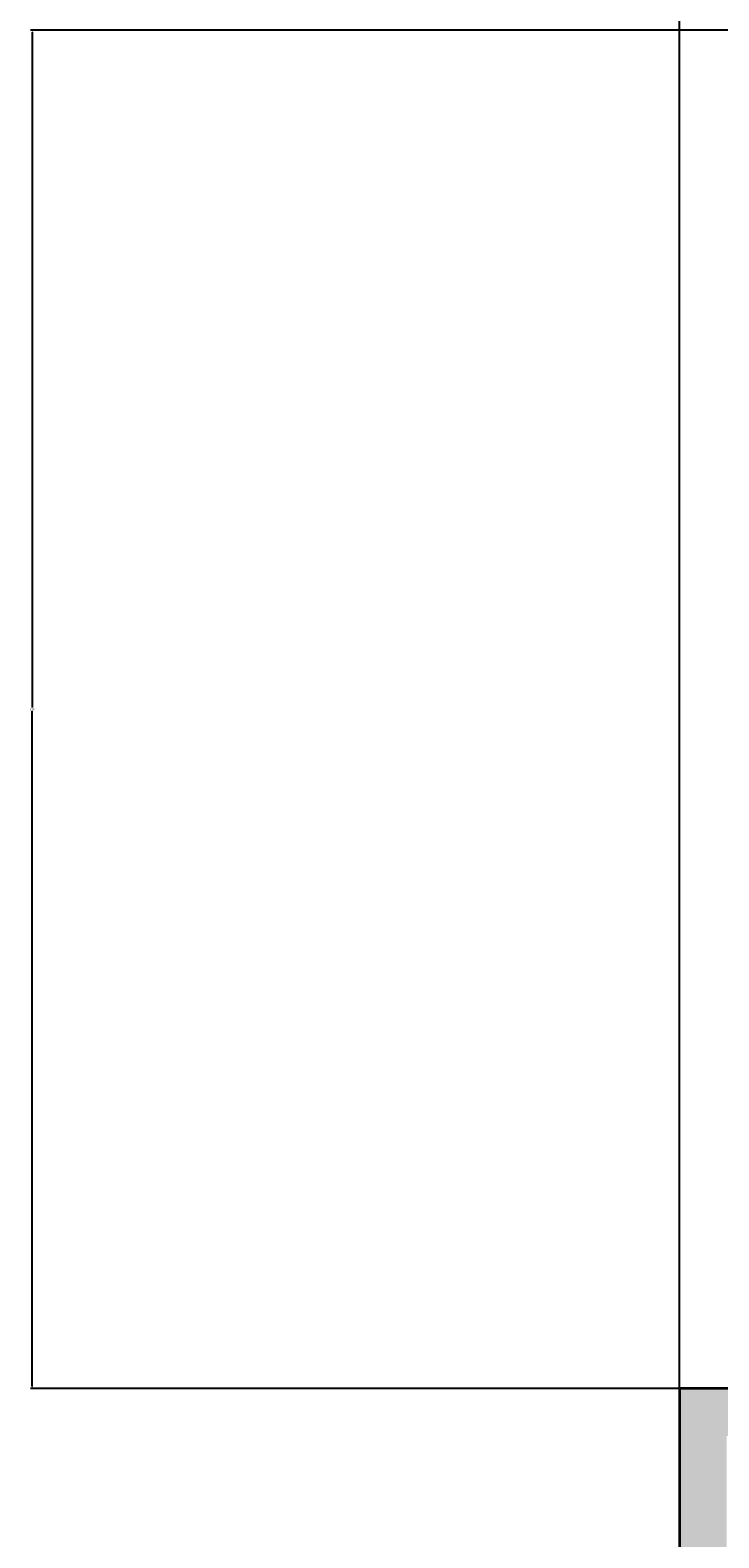
# Model space of a CAD drawing. Units: inches. Extents: x 1998 to 2588, y 1139 to 1977.
# Tile 58 of 134: x 1998 to 2063, y 1746 to 1889. Entities that reach past the tile are written whole.
import ezdxf

# ---------------------------------------------------------------- set-up
doc = ezdxf.new("R2010")
doc.units = ezdxf.units.IN
for name, color, linetype, lineweight in [('A-ANNO-DIMS', 2, 'Continuous', 18), ('A-WALL-PATT', 252, 'Continuous', 13), ('WALL', 200, 'Continuous', 35)]:
    doc.layers.add(name, color=color, linetype=linetype, lineweight=lineweight)
doc.styles.get("Standard").update_dxf_attribs({"font": 'arial.ttf'})
doc.dimstyles.get("Standard").update_dxf_attribs({"dimtxt": 0.18, "dimasz": 0.18, "dimexe": 0.18, "dimexo": 0.0625, "dimgap": 0.09, "dimtad": 0, "dimtih": 1, "dimtoh": 1, "dimdec": 4, "dimzin": 0, "dimdsep": 46, "dimtxsty": 'Standard', "dimcen": 0.09, "dimadec": 0, "dimazin": 0, "dimtfac": 1, "dimtdec": 4, "dimtofl": 0, "dimtmove": 0, "dimatfit": 3, "dimfxl": 1, "dimtolj": 1, "dimtzin": 0, "dimarcsym": 0})

# ---------------------------------------------------------------- blocks, each defined once
blk = doc.blocks.new('*D28')
at = {"layer": 'A-ANNO-DIMS', "color": 0, "lineweight": -2, "transparency": 16777216}
for p, q in [((2059.47, 1759.79), (2059.47, 1977.36)), ((2059.65, 1977.18), (2073.4, 1977.18)), ((2087.79, 1977.18), (2074.05, 1977.18)), ((2087.97, 1759.79), (2087.97, 1977.36))]:
    blk.add_line(p, q, dxfattribs=at)
at = {"layer": 'A-ANNO-DIMS', "color": 0, "transparency": 16777216}
for points in [[(2059.65, 1977.21), (2059.65, 1977.15), (2059.47, 1977.18)], [(2087.79, 1977.21), (2087.79, 1977.15), (2087.97, 1977.18)]]:
    blk.add_solid(points, dxfattribs=at)
at = {"layer": 'Defpoints', "color": 0, "transparency": 16777216}
for p in [(2087.97, 1977.18), (2059.47, 1759.73), (2087.97, 1759.73)]:
    blk.add_point(p, dxfattribs=at)
at = {"layer": 'A-ANNO-DIMS', "color": 0, "transparency": 16777216, "insert": (2073.72, 1977.18), "char_height": 0.18, "attachment_point": 5}
blk.add_mtext('\\A1;28.5', dxfattribs=at)
blk = doc.blocks.new('*D29')
at = {"layer": 'A-ANNO-DIMS', "color": 0, "lineweight": -2, "transparency": 16777216}
for p, q in [((2087.91, 1888.73), (1997.84, 1888.73)), ((1998.02, 1888.55), (1998.02, 1824.41)), ((1998.02, 1759.91), (1998.02, 1824.05)), ((2059.41, 1759.73), (1997.84, 1759.73))]:
    blk.add_line(p, q, dxfattribs=at)
at = {"layer": 'A-ANNO-DIMS', "color": 0, "transparency": 16777216}
for points in [[(1997.99, 1888.55), (1998.05, 1888.55), (1998.02, 1888.73)], [(1997.99, 1759.91), (1998.05, 1759.91), (1998.02, 1759.73)]]:
    blk.add_solid(points, dxfattribs=at)
at = {"layer": 'Defpoints', "color": 0, "transparency": 16777216}
for p in [(1998.02, 1888.73), (2087.97, 1888.73), (2059.47, 1759.73)]:
    blk.add_point(p, dxfattribs=at)
at = {"layer": 'A-ANNO-DIMS', "color": 0, "transparency": 16777216, "insert": (1998.02, 1824.23), "char_height": 0.18, "attachment_point": 5}
blk.add_mtext('\\A1;129', dxfattribs=at)

msp = doc.modelspace()

# ---------------------------------------------------------------- hatches: boundary and pattern name
at = {"layer": 'A-WALL-PATT'}
h = msp.add_hatch(color=256, dxfattribs=at)
h.dxf.hatch_style = 1
h.paths.add_polyline_path([(2222.9729, 1888.7324), (2099.4125, 1888.7324), (2099.4125, 1879.7324), (2222.9729, 1879.7324)])
h.paths.add_polyline_path([(2096.9729, 1868.3278), (2087.9729, 1868.3278), (2087.9729, 1775.637), (2096.9729, 1775.637)])
h.paths.add_polyline_path([(2227.4729, 1868.3278), (2222.9729, 1868.3278), (2222.9729, 1774.3318), (2227.4729, 1774.3318)])
h.paths.add_polyline_path([(2188.3019, 1759.7324), (2138.6074, 1759.7324), (2099.4125, 1759.7324), (2099.4125, 1755.2324), (2176.9729, 1755.2324), (2188.3019, 1755.2324)])
h.paths.add_polyline_path([(2087.9729, 1759.7324), (2059.4729, 1759.7324), (2059.4729, 1702.7324), (2087.9729, 1702.7324), (2087.9729, 1707.2324), (2063.9729, 1707.2324), (2063.9729, 1755.2324), (2087.9729, 1755.2324)])
h.paths.add_polyline_path([(2096.9729, 1755.2324), (2087.9729, 1755.2324), (2087.9729, 1707.2324), (2096.9729, 1707.2324)])
h.paths.add_polyline_path([(2187.0461, 1707.2324), (2105.9729, 1707.2324), (2096.9729, 1707.2324), (2087.9729, 1707.2324), (2087.9729, 1702.7324), (2105.9729, 1702.7324), (2114.9729, 1702.7324), (2187.0461, 1702.7324)])
h.paths.add_polyline_path([(2181.4729, 1719.2028), (2176.9729, 1719.2028), (2176.9729, 1707.2324), (2181.4729, 1707.2324)])
h.paths.add_polyline_path([(2216.0332, 1588.7324), (2114.9729, 1588.7324), (2105.9729, 1588.7324), (2105.9729, 1584.2324), (2216.0332, 1584.2324)])
h.paths.add_polyline_path([(2077.691, 1588.7324), (2061.4729, 1588.7324), (2061.4729, 1584.2324), (2077.691, 1584.2324)])
h.paths.add_polyline_path([(2105.9729, 1588.7324), (2098.0956, 1588.7324), (2098.0956, 1584.2324), (2105.9729, 1584.2324)])
h.paths.add_polyline_path([(2114.9729, 1596.2642), (2110.1012, 1596.2642), (2105.9729, 1596.2642), (2105.9729, 1588.7324), (2114.9729, 1588.7324)])
h.paths.add_polyline_path([(2114.9729, 1584.2324), (2105.9729, 1584.2324), (2105.9729, 1580.249), (2110.1012, 1580.249), (2114.9729, 1580.249)])
h.paths.add_polyline_path([(2114.9729, 1547.7716), (2110.1012, 1547.7716, -0.0318759), (2105.9729, 1548.035), (2105.9729, 1470.2324), (2108.3775, 1470.2324), (2108.3775, 1465.7324), (2186.2943, 1465.7324), (2186.2943, 1470.2324), (2114.9729, 1470.2324)])
h.paths.add_polyline_path([(2227.4729, 1584.2324), (2222.9729, 1584.2324), (2222.9729, 1486.137), (2227.4729, 1486.137)])
h.paths.add_polyline_path([(2295.4138, 1593.2324), (2227.4729, 1593.2324), (2227.4729, 1588.7324), (2295.4138, 1588.7324), (2295.4138, 1591.8729)])
h.paths.add_polyline_path([(2345.9729, 1627.1165), (2341.4729, 1627.1165), (2341.4729, 1593.2324), (2337.2869, 1593.2324), (2337.2869, 1591.8729), (2337.2869, 1588.7324), (2345.9729, 1588.7324)])
h.paths.add_polyline_path([(2291.9729, 1588.7324), (2287.4729, 1588.7324), (2287.4729, 1522.7324), (2291.9729, 1522.7324)])
h.paths.add_polyline_path([(2291.9729, 1522.7324), (2287.4729, 1522.7324), (2227.4729, 1522.7324), (2227.4729, 1518.2324), (2291.9729, 1518.2324)])
h.paths.add_polyline_path([(2295.7347, 1519.5919), (2295.7347, 1522.7324), (2291.9729, 1522.7324), (2291.9729, 1518.2324), (2295.7347, 1518.2324)])
h.paths.add_polyline_path([(2345.9729, 1522.7324), (2337.6078, 1522.7324), (2337.6078, 1519.5919), (2337.6078, 1518.2324), (2341.4729, 1518.2324), (2341.4729, 1488.5616), (2345.9729, 1488.5616)])
h.paths.add_polyline_path([(2345.9729, 1468.1569), (2341.4729, 1468.1569), (2341.4729, 1374.2324), (2227.4729, 1374.2324), (2227.4729, 1369.7324), (2345.9729, 1369.7324)])
h.paths.add_polyline_path([(2345.9729, 1369.7324), (2341.4729, 1369.7324), (2341.4729, 1362.2324), (2345.9729, 1362.2324)])
h.paths.add_polyline_path([(2345.9729, 1317.7324), (2345.9729, 1322.2324), (2341.4729, 1322.2324), (2341.4729, 1285.137), (2345.9729, 1285.137)], flags=17)
h.paths.add_polyline_path([(2356.2096, 1322.2324), (2345.9729, 1322.2324), (2345.9729, 1317.7324), (2356.2096, 1317.7324), (2356.2096, 1319.3088)], flags=17)
h.paths.add_polyline_path([(2393.9729, 1322.2324), (2375.6999, 1322.2324), (2375.6999, 1319.3088, -0.02024576), (2375.636, 1317.7324), (2393.9729, 1317.7324)], flags=17)
h.paths.add_polyline_path([(2398.4729, 1322.2324), (2393.9729, 1322.2324), (2393.9729, 1317.7324), (2393.9729, 1237.7324), (2345.9729, 1237.7324), (2345.9729, 1264.7324), (2341.4729, 1264.7324), (2341.4729, 1228.7324), (2393.9729, 1228.7324), (2482.7412, 1228.7324), (2482.7412, 1237.7324), (2398.4729, 1237.7324), (2398.4729, 1297.1029)])
h.paths.add_polyline_path([(2398.4729, 1362.2324), (2393.9729, 1362.2324), (2393.9729, 1357.7324), (2398.4729, 1357.7324)])
h.paths.add_polyline_path([(2345.9729, 1329.7549), (2341.4729, 1329.7549), (2341.4729, 1322.2324), (2345.9729, 1322.2324)])

# ---------------------------------------------------------------- linework, layer by layer
at = {"layer": 'WALL'}
for p, q in [((2087.9729, 1759.7324), (2059.4729, 1759.7324)), ((2059.4729, 1759.7324), (2059.4729, 1702.7324))]:
    msp.add_line(p, q, dxfattribs=at)

# ---------------------------------------------------------------- dimensions: what is measured, and where the dimension line sits
at = {"layer": 'A-ANNO-DIMS'}
dim = msp.add_linear_dim(base=(2087.9729, 1977.1824), p1=(2059.4729, 1759.7324), p2=(2087.9729, 1759.7324), dimstyle='Standard', override={"dimdec": 1, "dimlfac": 1, "dimrnd": 0, "dimzin": 0, "dimdsep": 46, "dimlunit": 2}, dxfattribs=at)
dim.commit()
dim.dimension.update_dxf_attribs({"geometry": '*D28', "text_midpoint": (2073.7229, 1977.1824)})
dim = msp.add_linear_dim(base=(1998.0229, 1888.7324), p1=(2059.4729, 1759.7324), p2=(2087.9729, 1888.7324), angle=90, dimstyle='Standard', override={"dimdec": 0, "dimlfac": 1, "dimrnd": 0, "dimzin": 0, "dimdsep": 46, "dimlunit": 2}, dxfattribs=at)
dim.commit()
dim.dimension.update_dxf_attribs({"geometry": '*D29', "text_midpoint": (1998.0229, 1824.2324)})

doc.saveas('drawing.dxf')
